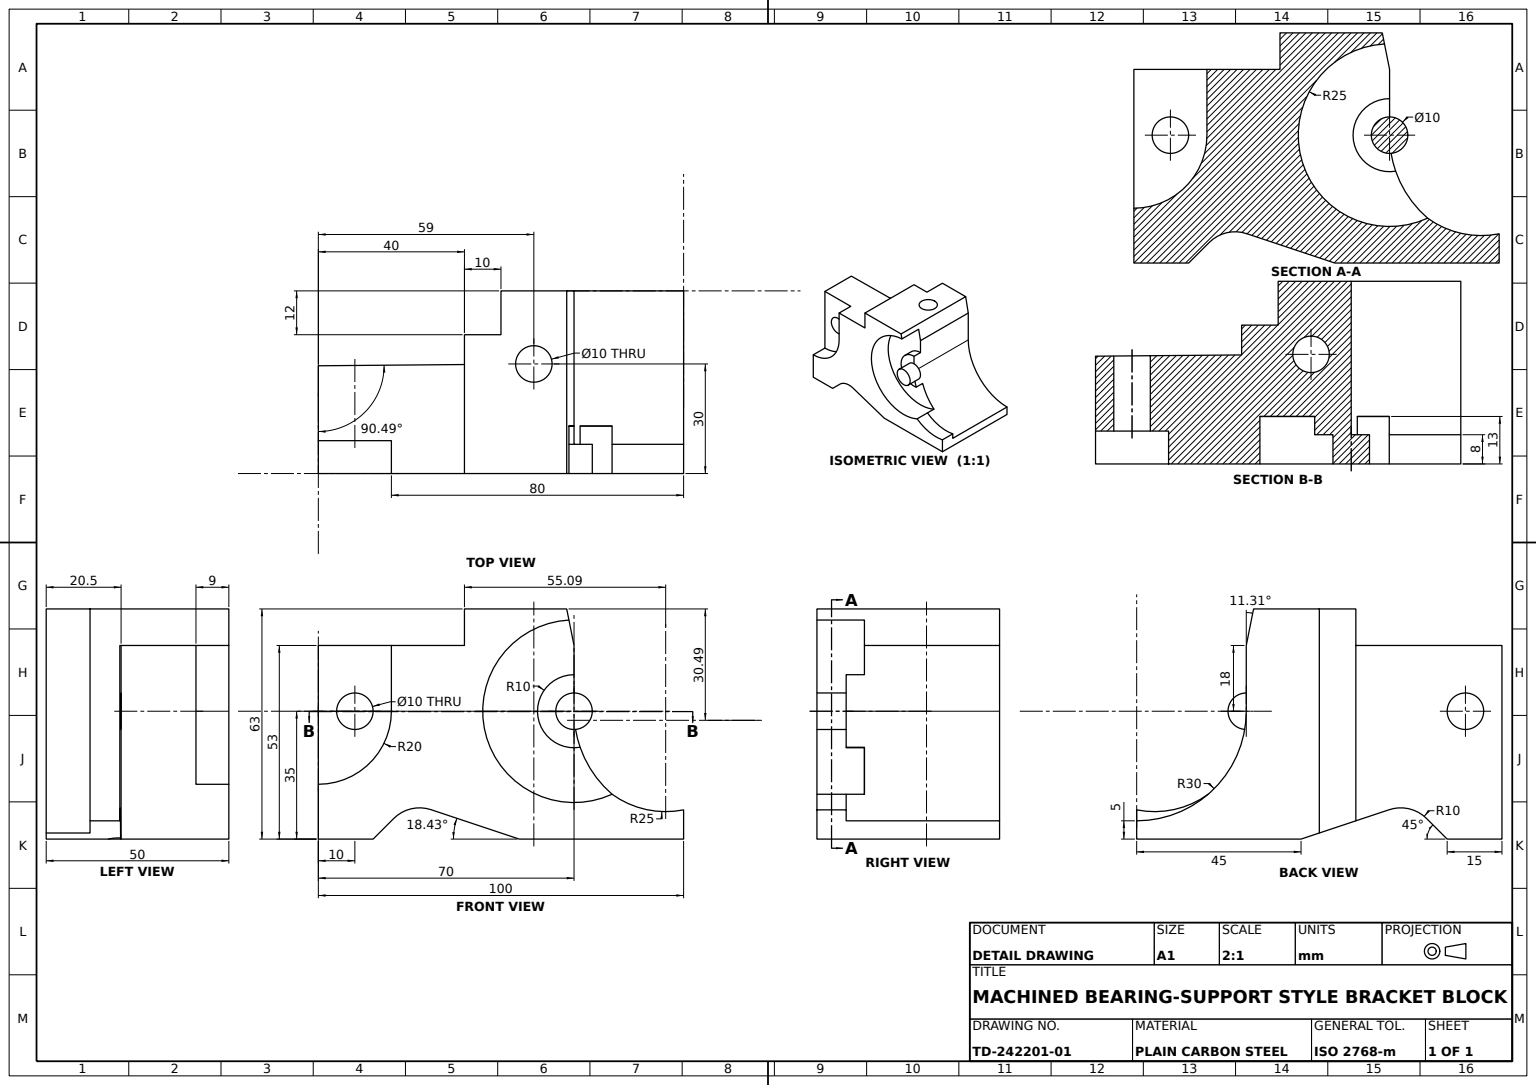
SolidWorks part; units mm, degrees
material "Plain Carbon Steel"
ref_plane "Front Plane" through (0, 0, 0) normal (0, 0, 1) x (1, 0, 0)
ref_plane "Top Plane" through (0, 0, 0) normal (0, 1, 0) x (1, 0, 0)
ref_plane "Right Plane" through (0, 0, 0) normal (1, 0, 0) x (0, 0, -1)
sketch "Block Profile Sketch" plane through (0, 0, 0) normal (0, 0, 1) x (1, 0, 0)
  line L0 (0, 0) -> (100, 0)
  line L1 (100, 0) -> (100, 5)
  line L2 (100, 0) -> (100, 5)
  line L3 (70, 53) -> (68, 63)
  line L4 (68, 63) -> (50, 63)
  line L5 (50, 63) -> (40, 63)
  line L6 (40, 63) -> (40, 53)
  line L7 (40, 53) -> (0, 53)
  line L8 (0, 53) -> (0, 0)
  line L9 (70, 35) -> (70, 53)
  arc A0 (70, 35) -> (100, 5) centre (100, 35) ccw
  dimension "D1" = 30
  dimension "D2" = 100
  dimension "D3" = 5
  dimension "D4" = 53
  dimension "D5" = 40
  dimension "D6" = 10
  dimension "D7" = 10
  dimension "D8" = 18
extrude "Block Body" add sketch "Block Profile Sketch" along normal blind 50 contours A0 L9 L3 L4 L5 L6 L7 L8 L0 L1
sketch "Bearing Arc Recess Sketch" plane through (0, 0, 50) normal (0, 0, 1) x (1, 0, 0)
  line L0 (40, 63) -> (40, 53) construction
  line L1 (68, 63) -> (40, 63) construction
  circle A0 centre (70, 35) radius 25
  circle A1 centre (70, 35) radius 10
  circle A2 centre (70, 35) radius 5
  arc M1 (100, 5) -> (70, 35) centre (100, 35) cw
  line M2 (70, 35) -> (70, 53)
  line M3 (70, 53) -> (68, 63)
  dimension "D1" = 25
  dimension "D2" = 10
  dimension "D3" = 10
  dimension "D4" = 30
  dimension "D5" = 28
extrude "Bearing Arc Recess" cut sketch "Bearing Arc Recess Sketch" against normal blind 13 contours A1 A0 M2 M3 M1
sketch "Arc Pocket Sketch" plane through (0, 0, 50) normal (0, 0, 1) x (1, 0, 0)
  circle A0 centre (70, 35) radius 10.0348
  circle A1 centre (70, 35) radius 5
  dimension "D1" = 20.0695
  dimension "D2" = 10
  dimension "D3" = 70
  dimension "D4" = 35
extrude "Arc Pocket" cut sketch "Arc Pocket Sketch" against normal blind 8
sketch "Pin Ø10 Sketch" plane through (0, 0, 50) normal (0, 0, 1) x (1, 0, 0)
  circle A0 centre (70, 35) radius 5
  dimension "D1" = 10
  dimension "D2" = 70
  dimension "D3" = 35
extrude "Pin Ø10" add sketch "Pin Ø10 Sketch" against normal blind 8
sketch "Side Boss Sketch" plane through (0, 0, 50) normal (0, 0, 1) x (1, 0, 0)
  line L0 (80.4167, 12.2735) -> (80.4167, 0)
  line L1 (80.4167, 0) -> (100, 0)
  line L2 (100, 0) -> (100, 8)
  line L3 (40, 63) -> (40, 53) construction
  line L4 (68, 63) -> (40, 63) construction
  arc A0 (80.4167, 12.2735) -> (100, 8) centre (95.0914, 32.5134) ccw
  dimension "D1" = 25
  dimension "D2" = 40.4167
  dimension "D3" = 55.0914
  dimension "D4" = 60
  dimension "D5" = 30.4866
  dimension "D6" = 63
extrude "Side Boss" add sketch "Side Boss Sketch" against normal blind 8
sketch "Profile Relief Sketch" plane through (0, 0, 50) normal (0, 0, 1) x (1, 0, 0)
  line L0 (0, 0) -> (15, 0)
  line L1 (15, 0) -> (55, 0)
  line L2 (15, 0) -> (25, 0)
  line L4 (15, 0) -> (20.6298, 5.6298)
  line L5 (55, 0) -> (30.8632, 8.0456)
  line L6 (100, 0) -> (100, 8) construction
  line L7 (0, 0) -> (100, 0) construction
  arc A0 (20.6298, 5.6298) -> (30.8632, 8.0456) centre (27.7009, -1.4412) cw
  spline S0 degree 1 poles (15, 0) (55, 0) knots 0 0 1 1
  line M2 (0, 0) -> (100, 0)
  dimension "D1" = 10
  dimension "D2" = 45
  dimension "D3" = 69.1368
  dimension "D4" = 72.2991
  dimension "D5" = 75
  dimension "D6" = 8.0456
  dimension "D8" = 100
extrude "Profile Relief Cut" cut sketch "Profile Relief Sketch" against normal through all contours A0 L4 L1 L5 M2
sketch "Step Cut Sketch" plane through (0, 0, 50) normal (0, 0, 1) x (1, 0, 0)
  line L0 (70, 35) -> (0, 35)
  line L1 (100, 0) -> (100, 8) construction
  line L2 (20, 35) -> (20, 53)
  line L3 (55, 0) -> (100, 0) construction
  circle A0 centre (0, 35) radius 20
  line M9 (40, 53) -> (0, 53)
  line M10 (0, 53) -> (0, 0)
  dimension "D1" = 20
  dimension "D2" = 30
  dimension "D3" = 80
  dimension "D4" = 35
  dimension "D5" = 53
extrude "Step Cut" cut sketch "Step Cut Sketch" against normal blind 9 contours L0 A0 M9 M10 | A0 L2 M9 | A0 L0 M10
sketch "Step Notch Sketch" plane through (0, 0, 41) normal (0, 0, 1) x (1, 0, 0)
  line L0 (0, 53) -> (10, 53)
  line L1 (20, 35) -> (10, 35)
  line L2 (10, 35) -> (10, 53)
  line L3 (0, 53) -> (0, 15) construction
  circle A0 centre (10, 35) radius 5
  dimension "D1" = 5
  dimension "D2" = 10
  dimension "D3" = 20
  dimension "D4" = 18
extrude "Step Notch" cut sketch "Step Notch Sketch" against normal through all contours L2 A0 L1 | L1 A0 L2
sketch "Slot Cut Sketch" plane through (0, 63, 0) normal (0, 1, 0) x (1, 0, 0)
  line L0 (68, 0) -> (59, 0)
  line L1 (59, -50) -> (59, -20)
  circle A0 centre (59, -20) radius 5
  dimension "D1" = 5
  dimension "D2" = 68
  dimension "D3" = 9
  dimension "D4" = 20
  dimension "D5" = 30
extrude "Slot Cut" cut sketch "Slot Cut Sketch" against normal through all
sketch "Top Relief Sketch" plane through (0, 63, 0) normal (0, 1, 0) x (1, 0, 0)
  line L0 (40, 0) -> (50, 0)
  line L1 (50, 0) -> (50, -12)
  line L2 (50, -12) -> (40, -12)
  line L3 (40, -12) -> (40, 0)
  line L4 (40, 0) -> (0, 0)
  line L5 (59, -20) -> (0, -20.5)
  line L6 (0, -20.5) -> (0, 0)
  line L7 (40, 0) -> (40, -20.161)
  line M2 (68, 0) -> (40, 0)
  line M3 (40, 0) -> (40, -50)
  dimension "D1" = 40
  dimension "D2" = 10
  dimension "D3" = 12
  dimension "D4" = 20.5
  dimension "D5" = 59
  dimension "D6" = 20
extrude "Top Relief Cut" cut sketch "Top Relief Sketch" against normal through all both and the other way through all contours L2 L1 M2 M3 | L6 L5 L4 M3
